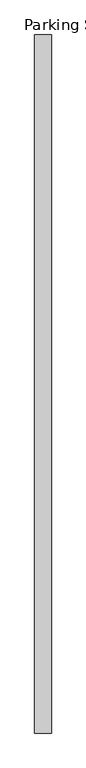
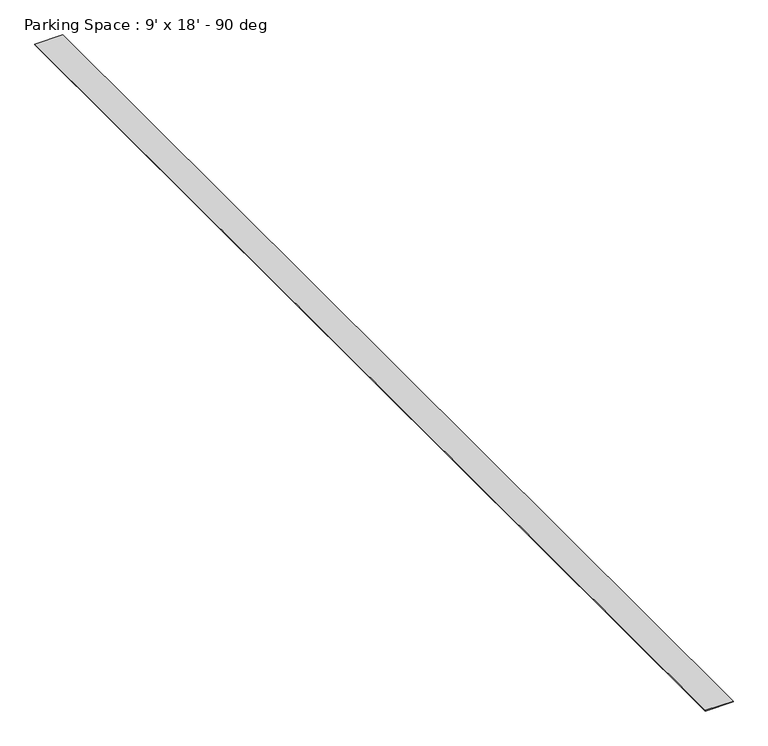
"""IFC4 building model written with IfcOpenShell, lengths in millimetres: proxy geometry, Parking Space : 9' x 18' - 90 deg."""

from ifc_helpers import new_model, si_unit, origin, origin_with_axes, place, context, project, spatial, polyline, outline, extrude, source, transform, mapped, element, save


def parking_space_9_x_18_90_deg_fdd9e8f5(model_context):
    return source(origin(), model_context, "Body", "SweptSolid", [
        extrude(outline(polyline([(-50.8, 0.0), (50.8, 0.0), (50.8, -4267.2), (-50.8, -4267.2), (-50.8, 0.0)])), origin_with_axes(), (0.0, 0.0, 1.0), 3.175),
    ])


if __name__ == "__main__":
    model = new_model("IFC4")
    model_context = context("Model", 3, world=origin())
    ifc_project = project(units=[si_unit("LENGTHUNIT", "METRE", prefix="MILLI")], contexts=[model_context])
    site = spatial("IfcSite", under=ifc_project)
    building = spatial("IfcBuilding", under=site)
    placement = place(None, origin())
    parking_space_9_x_18_90_deg_shape = parking_space_9_x_18_90_deg_fdd9e8f5(model_context)
    element("IfcBuildingElementProxy", 1, Name="Parking Space : 9' x 18' - 90 deg", ObjectType="Parking Space : 9' x 18' - 90 deg", at=placement, inside=building, context=model_context, shape_type="MappedRepresentation", body=[
        mapped(parking_space_9_x_18_90_deg_shape, transform((0.0, 0.0, 0.0), x_axis=(1.0, 0.0, 0.0), y_axis=(0.0, 1.0, 0.0), z_axis=(0.0, 0.0, 1.0))),
    ])
    save(model, "model.ifc")

# Revit data of these elements
# Type "Parking Space : 9' x 18' - 90 deg"
#   Angle = 90.00°
#   Parking Length = 18' - 0"
#   Parking Width = 9' - 0"
#   pl = 14' - 0"
#   pw = 6' - 5"
# Element 1 (IfcBuildingElementProxy, "Parking Space : 9' x 18' - 90 deg")
#   Materials on its faces: "Parking Stripe"
# Materials
#   "Parking Stripe": class "Paint", colour RGB 250 250 91, transparency 0
